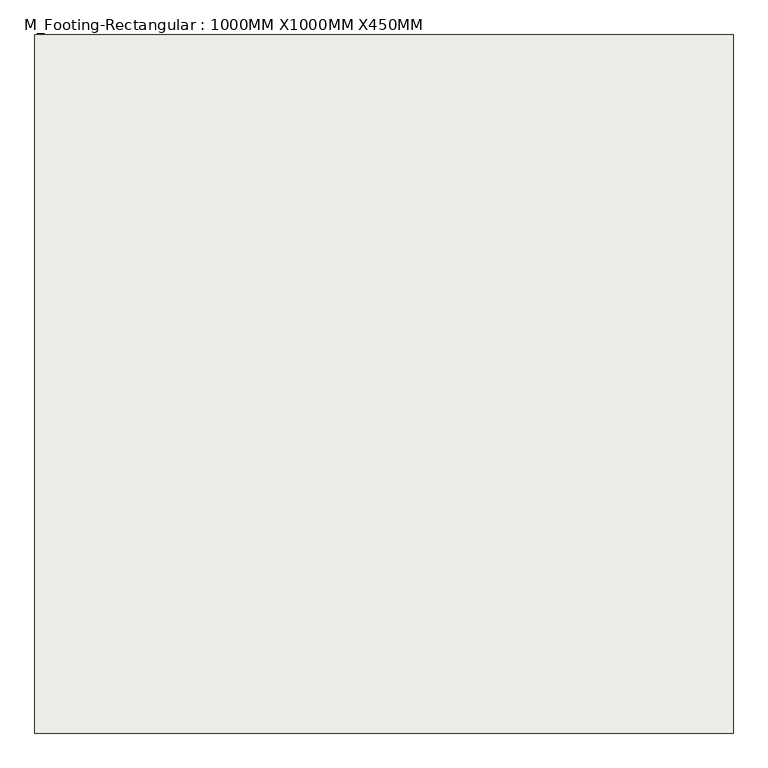
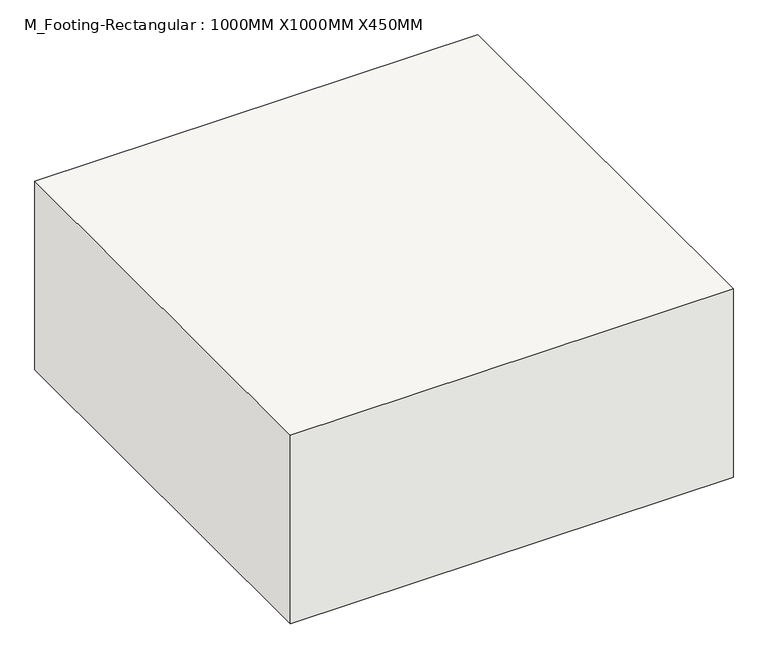
"""IFC4 building model written with IfcOpenShell, lengths in millimetres: slab geometry, M_Footing-Rectangular : 1000MM X1000MM X450MM."""

from ifc_helpers import new_model, si_unit, frame, origin, place, context, project, spatial, polyline, outline, extrude, source, transform, mapped, element, save


def m_footing_rectangular_1000mm_x1000mm_x450mm_4c97ae35(model_context):
    return source(origin(), model_context, "Body", "SweptSolid", [
        extrude(outline(polyline([(500.0, 500.0), (500.0, -500.0), (-500.0, -500.0), (-500.0, 500.0), (500.0, 500.0)])), frame((0.0, 0.0, -450.0), z_axis=(0.0, 0.0, 1.0), x_axis=(1.0, 0.0, 0.0)), (0.0, 0.0, 1.0), 450.0),
    ])


if __name__ == "__main__":
    model = new_model("IFC4")
    model_context = context("Model", 3, world=origin())
    ifc_project = project(units=[si_unit("LENGTHUNIT", "METRE", prefix="MILLI")], contexts=[model_context])
    site = spatial("IfcSite", under=ifc_project)
    building = spatial("IfcBuilding", under=site)
    placement = place(None, origin())
    m_footing_rectangular_1000mm_x1000mm_x450mm_shape = m_footing_rectangular_1000mm_x1000mm_x450mm_4c97ae35(model_context)
    element("IfcSlab", 1, ObjectType="M_Footing-Rectangular : 1000MM X1000MM X450MM", at=placement, inside=building, context=model_context, shape_type="MappedRepresentation", body=[
        mapped(m_footing_rectangular_1000mm_x1000mm_x450mm_shape, transform((0.0, 0.0, 0.0), x_axis=(1.0, 0.0, 0.0), y_axis=(0.0, 1.0, 0.0), z_axis=(0.0, 0.0, 1.0))),
    ])
    save(model, "model.ifc")

# Revit data of these elements
# Type "M_Footing-Rectangular : 1000MM X1000MM X450MM"
#   Width = 1000 mm
#   Length = 1000 mm
#   Foundation Thickness = 450 mm
#   Structural Material [instance default] = Concrete, Cast-in-Place gray
#   Assembly Code = ""
# Element 1 (IfcSlab, "M_Footing-Rectangular : 1000MM X1000MM X450MM")
#   Materials on its faces: "Concrete, Cast-in-Place gray"
# Materials
#   "Concrete, Cast-in-Place gray": class "Concrete", colour RGB 192 192 192, transparency 0, Description = "Cast-in-place concrete", Cost = 0
